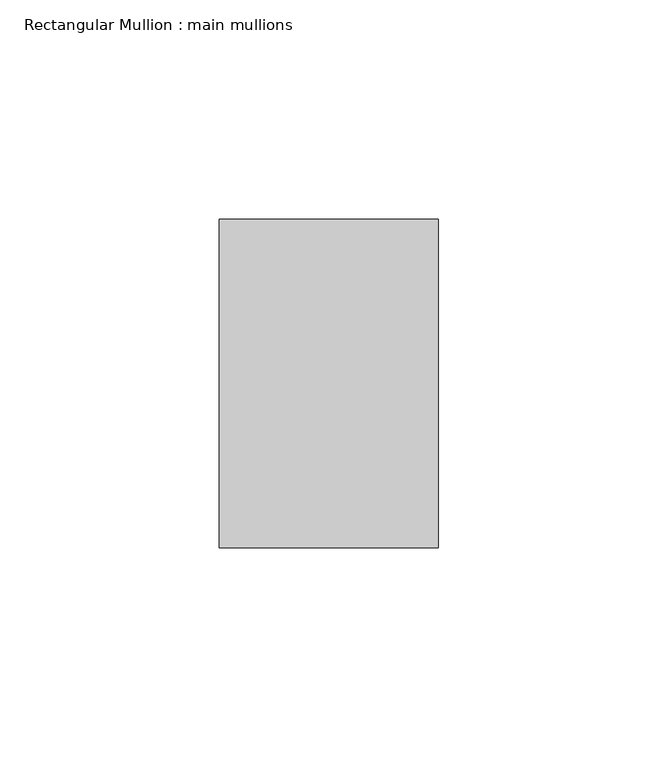
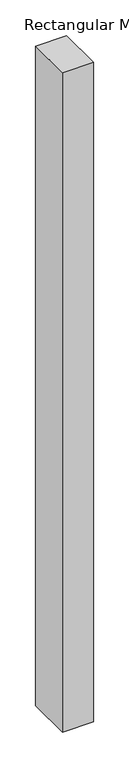
"""IFC4 building model written with IfcOpenShell, lengths in millimetres: member geometry, Rectangular Mullion : main mullions."""

from ifc_helpers import new_model, si_unit, frame, origin, place, context, project, spatial, polyline, outline, extrude, source, transform, mapped, element, save


def rectangular_mullion_main_mullions_1ff2eda8(model_context):
    return source(origin(), model_context, "Body", "SweptSolid", [
        extrude(outline(polyline([(0.0, 37.5), (0.0, -37.5), (-50.0, -37.5), (-50.0, 37.5), (0.0, 37.5)])), frame((0.0, 0.0, -1125.0), z_axis=(0.0, 0.0, 1.0), x_axis=(1.0, 0.0, 0.0)), (0.0, 0.0, 1.0), 1125.0),
    ])


if __name__ == "__main__":
    model = new_model("IFC4")
    model_context = context("Model", 3, world=origin())
    ifc_project = project(units=[si_unit("LENGTHUNIT", "METRE", prefix="MILLI")], contexts=[model_context])
    site = spatial("IfcSite", under=ifc_project)
    building = spatial("IfcBuilding", under=site)
    placement = place(None, origin())
    rectangular_mullion_main_mullions_shape = rectangular_mullion_main_mullions_1ff2eda8(model_context)
    element("IfcMember", 1, ObjectType="Rectangular Mullion : main mullions", at=placement, inside=building, context=model_context, shape_type="MappedRepresentation", body=[
        mapped(rectangular_mullion_main_mullions_shape, transform((0.0, 0.0, 0.0), x_axis=(1.0, 0.0, 0.0), y_axis=(0.0, 1.0, 0.0), z_axis=(0.0, 0.0, 1.0))),
    ])
    save(model, "model.ifc")

# Revit data of these elements
# Type "Rectangular Mullion : main mullions"
#   built-in parameter 1007304 = 0.246063 (stored number, unit not read)
#   built-in parameter 1007301 = 0.082021 (stored number, unit not read)
#   built-in parameter 1007300 = 0.082021 (stored number, unit not read)
# Element 1 (IfcMember, "Rectangular Mullion : main mullions")
#   Materials on its faces: "Aluminum"
# Materials
#   "Aluminum": class "Metal", colour RGB 136 136 136, transparency 0, Description = "Aluminum 6061", Cost = 0
